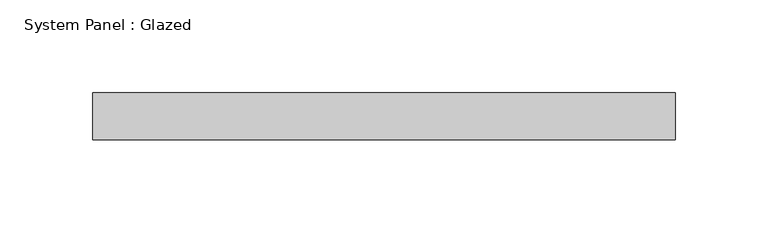
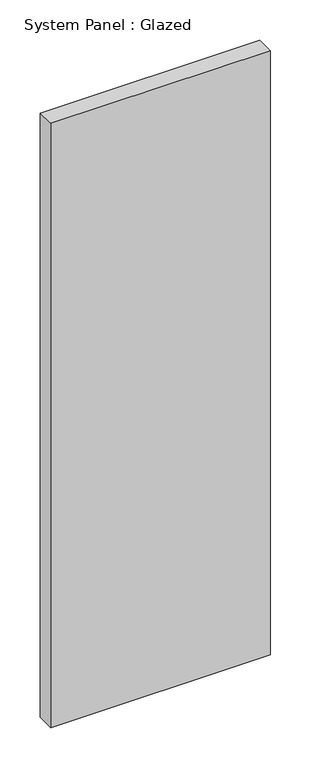
"""IFC4 building model written with IfcOpenShell, lengths in millimetres: plate geometry, System Panel : Glazed."""

from ifc_helpers import new_model, si_unit, origin, origin_with_axes, place, context, project, spatial, polyline, outline, extrude, source, transform, mapped, element, save


def system_panel_glazed_ca107f82(model_context):
    return source(origin(), model_context, "Body", "SweptSolid", [
        extrude(outline(polyline([(157.1014524, 19.05), (-157.1014524, 19.05), (-157.1014524, 44.45), (157.1014524, 44.45), (157.1014524, 19.05)])), origin_with_axes(), (0.0, 0.0, 1.0), 914.4),
    ])


if __name__ == "__main__":
    model = new_model("IFC4")
    model_context = context("Model", 3, world=origin())
    ifc_project = project(units=[si_unit("LENGTHUNIT", "METRE", prefix="MILLI")], contexts=[model_context])
    site = spatial("IfcSite", under=ifc_project)
    building = spatial("IfcBuilding", under=site)
    placement = place(None, origin())
    system_panel_glazed_shape = system_panel_glazed_ca107f82(model_context)
    element("IfcPlate", 1, ObjectType="System Panel : Glazed", at=placement, inside=building, context=model_context, shape_type="MappedRepresentation", body=[
        mapped(system_panel_glazed_shape, transform((0.0, 0.0, 0.0), x_axis=(1.0, 0.0, 0.0), y_axis=(0.0, 1.0, 0.0), z_axis=(0.0, 0.0, 1.0))),
    ])
    save(model, "model.ifc")

# Revit data of these elements
# Type "System Panel : Glazed"
#   Construction Type Id = "GSP4R"
#   Analytic Construction = "1/8 in Pilkington single glazing"
#   Visual Light Transmittance = 0.9
#   Solar Heat Gain Coefficient = 0.86
#   Heat Transfer Coefficient (U) = 1.18115 BTU/(h·ft²·°F)
# Element 1 (IfcPlate, "System Panel : Glazed")
#   Materials on its faces: "Glass"
# Materials
#   "Glass": class "Glass", colour RGB 0 128 192, transparency 0.75, Description = "Soda Lime Glass", Cost = 0
